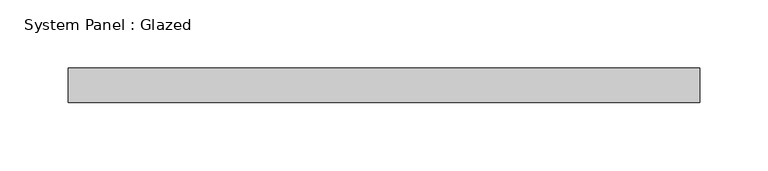
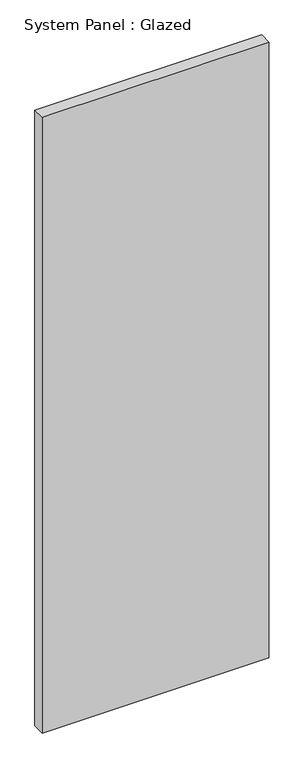
"""IFC4 building model written with IfcOpenShell, lengths in millimetres: plate geometry, System Panel : Glazed."""

from ifc_helpers import new_model, si_unit, origin, origin_with_axes, place, context, project, spatial, polyline, outline, extrude, source, transform, mapped, element, save


def system_panel_glazed_59e6c1d1(model_context):
    return source(origin(), model_context, "Body", "SweptSolid", [
        extrude(outline(polyline([(231.775, 19.05), (-231.775, 19.05), (-231.775, 44.45), (231.775, 44.45), (231.775, 19.05)])), origin_with_axes(), (0.0, 0.0, 1.0), 1330.6985165),
    ])


if __name__ == "__main__":
    model = new_model("IFC4")
    model_context = context("Model", 3, world=origin())
    ifc_project = project(units=[si_unit("LENGTHUNIT", "METRE", prefix="MILLI")], contexts=[model_context])
    site = spatial("IfcSite", under=ifc_project)
    building = spatial("IfcBuilding", under=site)
    placement = place(None, origin())
    system_panel_glazed_shape = system_panel_glazed_59e6c1d1(model_context)
    element("IfcPlate", 1, ObjectType="System Panel : Glazed", at=placement, inside=building, context=model_context, shape_type="MappedRepresentation", body=[
        mapped(system_panel_glazed_shape, transform((0.0, 0.0, 0.0), x_axis=(1.0, 0.0, 0.0), y_axis=(0.0, 1.0, 0.0), z_axis=(0.0, 0.0, 1.0))),
    ])
    save(model, "model.ifc")

# Revit data of these elements
# Type "System Panel : Glazed"
#   Construction Type Id = "GSP4R"
#   Analytic Construction = "1/8 in Pilkington single glazing"
#   Visual Light Transmittance = 0.9
#   Solar Heat Gain Coefficient = 0.86
#   Heat Transfer Coefficient (U) = 1.18115 BTU/(h·ft²·°F)
#   Define Thermal Properties by = 1
# Element 1 (IfcPlate, "System Panel : Glazed")
#   Materials on its faces: "Glass"
# Materials
#   "Glass": class "Glass", colour RGB 0 128 192, transparency 0.75, Description = "Soda Lime Glass", Cost = 0
